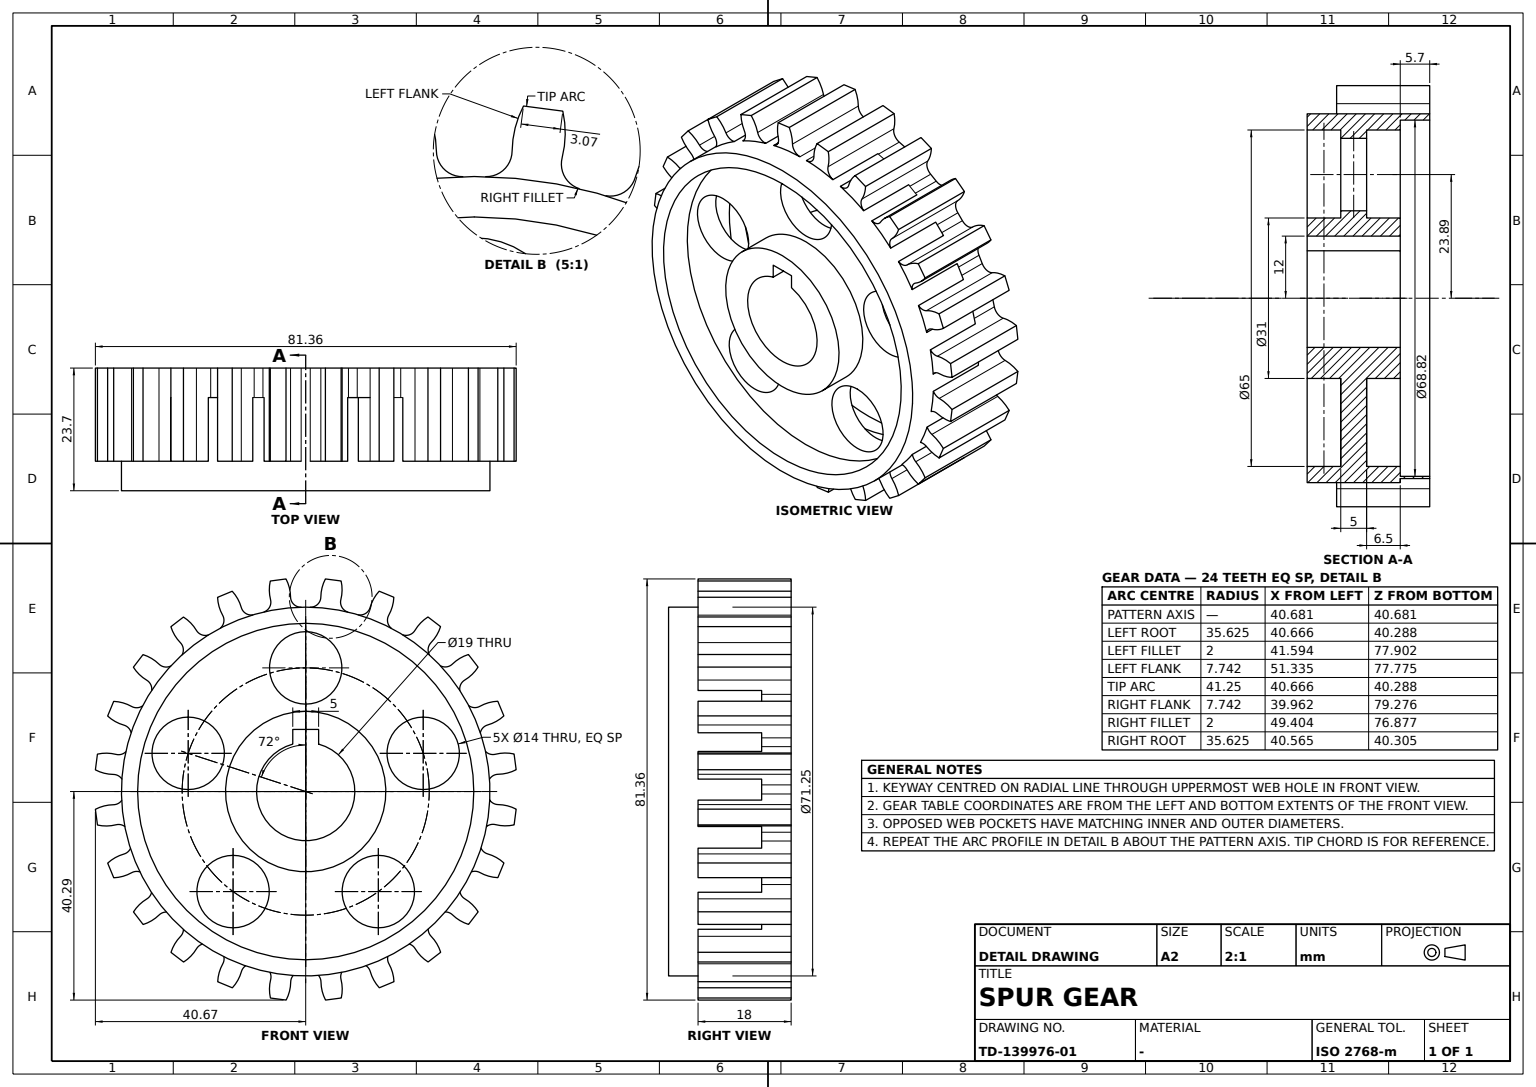
CATIA V5 part; units mm, degrees
sketch "Sketch1" plane through (0, 0, 0) normal (0, 1, 0) x (-1, 0, 0)
  point P0 (0, 9.5)
  line L0 (0, 9.5) -> (-5.7, 9.5)
  line L1 (-5.7, 9.5) -> (-5.7, 15.5)
  line L2 (-5.7, 15.5) -> (0.8, 15.5)
  line L3 (0.8, 15.5) -> (0.8, 32.5)
  line L4 (0.8, 32.5) -> (-5.7, 32.5)
  point P1 (-5.7, 32.5)
  line L5 (-5.7, 32.5) -> (-5.7, 35.625)
  line L6 (-5.7, 35.625) -> (12.3, 35.625)
  line L7 (12.3, 35.625) -> (12.3, 32.5)
  point P2 (12.3, 32.5)
  line L8 (12.3, 32.5) -> (5.8, 32.5)
  line L9 (5.8, 32.5) -> (5.8, 15.5)
  point P3 (5.8, 15.5)
  line L10 (5.8, 15.5) -> (12.3, 15.5)
  point P4 (12.3, 15.5)
  line L11 (12.3, 15.5) -> (12.3, 9.5)
  point P5 (12.3, 9.5)
  line L12 (12.3, 9.5) -> (0, 9.5)
  dimension "length L7" = 3.125
  dimension "length L11" = 6
  dimension "distance L1 y axis" = 5.7
  dimension "distance L3 L5" = 6.5
  dimension "distance L9 L3" = 5
  dimension "distance L5 L7" = 18
  dimension "distance L6 x axis" = 35.625
  dimension "distance L12 x axis" = 9.5
  constraint coincidence P0 y-axis
  constraint coincidence P1 L1
  constraint coincidence P2 L4
  constraint coincidence P3 L2
  constraint coincidence P4 L7
  constraint coincidence P5 L0
  constraint horizontal L0 x-axis
  constraint horizontal L2 x-axis
  constraint horizontal L4 x-axis
  constraint horizontal L6 x-axis
  constraint horizontal L8 x-axis
  constraint horizontal L10 x-axis
  constraint horizontal L12 x-axis
  constraint vertical L1 y-axis
  constraint vertical L3 y-axis
  constraint vertical L5 y-axis
  constraint vertical L7 y-axis
  constraint vertical L9 y-axis
  constraint vertical L11 y-axis
revolve "Shaft1" add sketch "Sketch1" angle 360 about axis through (0, 0, 0) along (-1, 0, 0)
sketch "Sketch2" plane through (0, 0, 0) normal (1, 0, 0) x (0, 1, 0)
  circle A0 centre (0, 23.89) radius 7
  point P0 (0, 23.89)
  circle A1 centre (-22.7207, 7.3824) radius 7
  circle A2 centre (-14.0422, -19.3274) radius 7
  circle A3 centre (14.0422, -19.3274) radius 7
  circle A4 centre (22.7207, 7.3824) radius 7
  circle A5 centre (0, 0) radius 9.5 construction
  arc A6 (2.5, 9.1652) -> (-2.5, 9.1652) centre (0, 0) ccw
  line L0 (-2.5, 12) -> (2.5, 12)
  line L1 (2.5, 12) -> (2.5, 9.1652)
  line L2 (-2.5, 9.1652) -> (-2.5, 12)
  point P1 (-2.5, 9.1652)
  dimension "radius A0" = 7
  dimension "distance P0 x axis" = 23.89
  dimension "distance L0 x axis" = 12
  dimension "length L0" = 5
  constraint coincidence P0 y-axis
  constraint coincidence P1 A5
  constraint horizontal L0 x-axis
  constraint vertical L1 y-axis
  constraint vertical L2 y-axis
  constraint symmetry L2 L1 y-axis
extrude "Pocket1" cut sketch "Sketch2" against normal through all and the other way up to next
sketch "Sketch3" plane through (0, 0, 0) normal (1, 0, 0) x (0, 1, 0)
  circle A0 centre (0, 0) radius 35.625 construction
  arc A1 (0.8787, 35.6142) -> (-0.8787, 35.6142) centre (0, 0) ccw
  circle A2 centre (0, 0) radius 34.411
  arc A3 (-2.9279, 37.5875) -> (-3.8084, 41.0738) centre (-10.669, 37.4868) ccw
  point P0 (-2.5164, 34.3189)
  point P1 (-6.4518, 33.8008)
  point P2 (-3.8084, 41.0738)
  point P3 (6.8509, 40.6771)
  point P4 (3.8084, 41.0738)
  arc A4 (3.8084, 41.0738) -> (6.8509, 40.6771) centre (0, 0) cw
  arc A5 (2.9279, 37.5875) -> (3.8084, 41.0738) centre (10.669, 37.4868) cw
  point P5 (-3.1914, 35.4818)
  point P6 (3.1914, 35.4818)
  arc A6 (-2.9279, 37.5875) -> (-0.8787, 35.6142) centre (-0.9281, 37.6136) ccw
  arc A7 (2.9279, 37.5875) -> (0.8787, 35.6142) centre (0.9281, 37.6136) cw
  point P7 (40.2989, -6.4434)
  point P8 (37.1569, -16.6368)
  point P9 (35.0987, -6.1007)
  point P10 (33.4468, -12.266)
  arc A8 (36.7035, -6.3916) -> (40.2989, -6.4434) centre (38.6097, 1.1119) ccw
  arc A9 (38.3275, -13.8006) -> (37.1569, -16.6368) centre (-0.3611, 0.5087) cw
  arc A10 (35.1879, -12.0478) -> (38.3275, -13.8006) centre (33.087, -19.4991) cw
  arc A11 (36.7035, -6.3916) -> (34.267, -7.8602) centre (36.211, -8.33) ccw
  arc A12 (35.1879, -12.0478) -> (33.8121, -9.5577) centre (35.7306, -10.1229) cw
  circle A13 centre (0, 0) radius 35.625 construction
  arc A14 (33.8121, -9.5577) -> (34.267, -7.8602) centre (-0.3611, 0.5087) ccw
  point P11 (-17.015, -36.7494)
  point P12 (-26.0479, -31.0762)
  point P13 (-14.9771, -32.3238)
  point P14 (-20.5047, -29.1324)
  arc A15 (-16.0344, -33.2899) -> (-17.015, -36.7494) centre (-9.28, -37.0732) ccw
  arc A16 (-23.6114, -32.941) -> (-26.0479, -31.0762) centre (0.2237, 0.7258) cw
  arc A17 (-21.1057, -30.362) -> (-23.6114, -32.941) centre (-27.7593, -26.4042) cw
  arc A18 (-16.0344, -33.2899) -> (-16.8224, -30.5563) centre (-17.7793, -32.3125) ccw
  arc A19 (-21.1057, -30.362) -> (-18.3444, -29.6776) centre (-19.3868, -31.3845) cw
  arc A20 (-18.3444, -29.6776) -> (-16.8224, -30.5563) centre (0.2237, 0.7258) ccw
  circle A21 centre (0, 0) radius 35.625 construction
  point P15 (-31.4544, 26.4554)
  point P16 (-23.6367, 33.7121)
  point P17 (-27.346, 22.8328)
  point P18 (-22.8328, 27.346)
  arc A22 (-28.3666, 24.6128) -> (-31.4544, 26.4554) centre (-33.7692, 19.0677) ccw
  arc A23 (-26.0686, 31.8412) -> (-23.6367, 33.7121) centre (0.2821, 0.1047) cw
  arc A24 (-24.226, 28.7535) -> (-26.0686, 31.8412) centre (-18.6809, 34.156) cw
  arc A25 (-28.3666, 24.6128) -> (-25.5223, 24.6664) centre (-26.971, 26.0453) ccw
  arc A26 (-24.226, 28.7535) -> (-24.2796, 25.9091) centre (-25.6585, 27.3578) cw
  arc A27 (-24.2796, 25.9091) -> (-25.5223, 24.6664) centre (0.2821, 0.1047) ccw
  circle A28 centre (0, 0) radius 35.625 construction
  point P19 (33.3339, 24.0442)
  point P20 (38.3199, 14.6146)
  point P21 (29.1324, 20.5047)
  point P22 (32.3238, 14.9771)
  arc A29 (30.7549, 21.5385) -> (33.3339, 24.0442) centre (26.7971, 28.1921) ccw
  arc A30 (37.1422, 17.4478) -> (38.3199, 14.6146) centre (-0.3329, 0.2091) cw
  arc A31 (33.6828, 16.4672) -> (37.1422, 17.4478) centre (37.4661, 9.7128) cw
  arc A32 (30.7549, 21.5385) -> (30.0705, 18.7772) centre (31.7773, 19.8196) ccw
  arc A33 (33.6828, 16.4672) -> (30.9492, 17.2552) centre (32.7054, 18.2121) cw
  arc A34 (30.9492, 17.2552) -> (30.0705, 18.7772) centre (-0.3329, 0.2091) ccw
  circle A35 centre (0, 0) radius 35.625 construction
  point P23 (14.2364, -37.9125)
  point P24 (3.8376, -40.2881)
  point P25 (12.266, -33.4468)
  point P26 (6.1007, -35.0987)
  arc A36 (12.4836, -34.7728) -> (14.2364, -37.9125) centre (19.9349, -32.672) ccw
  arc A37 (6.8791, -39.8838) -> (3.8376, -40.2881) centre (-0.0729, 0.7761) cw
  arc A38 (6.8273, -36.2884) -> (6.8791, -39.8838) centre (-0.6762, -38.1947) cw
  arc A39 (12.4836, -34.7728) -> (9.9935, -33.3971) centre (10.5586, -35.3156) ccw
  arc A40 (6.8273, -36.2884) -> (8.2959, -33.8519) centre (8.7657, -35.796) cw
  arc A41 (8.2959, -33.8519) -> (9.9935, -33.3971) centre (-0.0729, 0.7761) ccw
  circle A42 centre (0, 0) radius 35.625 construction
  point P27 (-40.6663, -3.4301)
  point P28 (-40.2696, 7.2291)
  point P29 (-35.4818, -3.1914)
  point P30 (-35.4818, 3.1914)
  arc A43 (-37.18, -2.5497) -> (-40.6663, -3.4301) centre (-37.0793, -10.2908) ccw
  arc A44 (-40.6663, 4.1866) -> (-40.2696, 7.2291) centre (0.4075, 0.3782) cw
  arc A45 (-37.18, 3.3061) -> (-40.6663, 4.1866) centre (-37.0793, 11.0473) cw
  arc A46 (-37.18, -2.5497) -> (-35.2067, -0.5005) centre (-37.2061, -0.5498) ccw
  arc A47 (-37.18, 3.3061) -> (-35.2067, 1.257) centre (-37.2061, 1.3063) cw
  arc A48 (-35.2067, 1.257) -> (-35.2067, -0.5005) centre (0.4075, 0.3782) ccw
  circle A49 centre (0, 0) radius 35.625 construction
  point P31 (6.8509, 40.6771)
  point P32 (17.0443, 37.5351)
  point P33 (6.1007, 35.0987)
  point P34 (12.266, 33.4468)
  arc A50 (6.7991, 37.0817) -> (6.8509, 40.6771) centre (-0.7044, 38.988) ccw
  arc A51 (14.2081, 38.7058) -> (17.0443, 37.5351) centre (-0.1012, 0.0172) cw
  arc A52 (12.4553, 35.5661) -> (14.2081, 38.7058) centre (19.9066, 33.4653) cw
  arc A53 (6.7991, 37.0817) -> (8.2676, 34.6452) centre (8.7375, 36.5893) ccw
  arc A54 (12.4553, 35.5661) -> (9.9652, 34.1904) centre (10.5304, 36.1089) cw
  arc A55 (9.9652, 34.1904) -> (8.2676, 34.6452) centre (-0.1012, 0.0172) ccw
  circle A56 centre (0, 0) radius 35.625 construction
  point P35 (37.1569, -16.6368)
  point P36 (31.4837, -25.6696)
  point P37 (32.3238, -14.9771)
  point P38 (29.1324, -20.5047)
  arc A57 (33.6974, -15.6562) -> (37.1569, -16.6368) centre (37.4807, -8.9018) ccw
  arc A58 (33.3485, -23.2331) -> (31.4837, -25.6696) centre (-0.3183, 0.602) cw
  arc A59 (30.7695, -20.7274) -> (33.3485, -23.2331) centre (26.8117, -27.3811) cw
  arc A60 (33.6974, -15.6562) -> (30.9638, -16.4441) centre (32.72, -17.4011) ccw
  arc A61 (30.7695, -20.7274) -> (30.0851, -17.9661) centre (31.792, -19.0085) cw
  arc A62 (30.0851, -17.9661) -> (30.9638, -16.4441) centre (-0.3183, 0.602) ccw
  circle A63 centre (0, 0) radius 35.625 construction
  point P39 (-26.0479, -31.0762)
  point P40 (-33.3046, -23.2584)
  point P41 (-22.8328, -27.346)
  point P42 (-27.346, -22.8328)
  arc A64 (-24.2053, -27.9884) -> (-26.0479, -31.0762) centre (-18.6602, -33.391) ccw
  arc A65 (-31.4338, -25.6903) -> (-33.3046, -23.2584) centre (0.3028, 0.6603) cw
  arc A66 (-28.346, -23.8477) -> (-31.4338, -25.6903) centre (-33.7485, -18.3027) cw
  arc A67 (-24.2053, -27.9884) -> (-24.2589, -25.1441) centre (-25.6378, -26.5927) ccw
  arc A68 (-28.346, -23.8477) -> (-25.5016, -23.9013) centre (-26.9503, -25.2802) cw
  arc A69 (-25.5016, -23.9013) -> (-24.2589, -25.1441) centre (0.3028, 0.6603) ccw
  circle A70 centre (0, 0) radius 35.625 construction
  point P43 (-23.6367, 33.7121)
  point P44 (-14.2071, 38.6982)
  point P45 (-20.5047, 29.1324)
  point P46 (-14.9771, 32.3238)
  arc A71 (-21.131, 31.1331) -> (-23.6367, 33.7121) centre (-27.7847, 27.1753) ccw
  arc A72 (-17.0404, 37.5205) -> (-14.2071, 38.6982) centre (0.1984, 0.0453) cw
  arc A73 (-16.0597, 34.061) -> (-17.0404, 37.5205) centre (-9.3053, 37.8443) cw
  arc A74 (-21.131, 31.1331) -> (-18.3697, 30.4487) centre (-19.4121, 32.1556) ccw
  arc A75 (-16.0597, 34.061) -> (-16.8477, 31.3275) centre (-17.8047, 33.0836) cw
  arc A76 (-16.8477, 31.3275) -> (-18.3697, 30.4487) centre (0.1984, 0.0453) ccw
  circle A77 centre (0, 0) radius 35.625 construction
  point P47 (38.3199, 14.6146)
  point P48 (40.6956, 4.2159)
  point P49 (33.4468, 12.266)
  point P50 (35.0987, 6.1007)
  arc A78 (35.1803, 12.8618) -> (38.3199, 14.6146) centre (33.0794, 20.3131) ccw
  arc A79 (40.2913, 7.2574) -> (40.6956, 4.2159) centre (-0.3686, 0.3053) cw
  arc A80 (36.6959, 7.2055) -> (40.2913, 7.2574) centre (38.6022, -0.2979) cw
  arc A81 (35.1803, 12.8618) -> (33.8046, 10.3717) centre (35.7231, 10.9369) ccw
  arc A82 (36.6959, 7.2055) -> (34.2594, 8.6741) centre (36.2035, 9.144) cw
  arc A83 (34.2594, 8.6741) -> (33.8046, 10.3717) centre (-0.3686, 0.3053) ccw
  circle A84 centre (0, 0) radius 35.625 construction
  point P51 (3.8376, -40.2881)
  point P52 (-6.8216, -39.8914)
  point P53 (3.1914, -35.4818)
  point P54 (-3.1914, -35.4818)
  arc A85 (2.9571, -36.8018) -> (3.8376, -40.2881) centre (10.6983, -36.701) ccw
  arc A86 (-3.7791, -40.2881) -> (-6.8216, -39.8914) centre (0.0292, 0.7857) cw
  arc A87 (-2.8987, -36.8018) -> (-3.7791, -40.2881) centre (-10.6398, -36.701) cw
  arc A88 (2.9571, -36.8018) -> (0.908, -34.8284) centre (0.9573, -36.8278) ccw
  arc A89 (-2.8987, -36.8018) -> (-0.8495, -34.8284) centre (-0.8988, -36.8278) cw
  arc A90 (-0.8495, -34.8284) -> (0.908, -34.8284) centre (0.0292, 0.7857) ccw
  circle A91 centre (0, 0) radius 35.625 construction
  point P55 (-40.2696, 7.2291)
  point P56 (-37.1276, 17.4225)
  point P57 (-35.0987, 6.1007)
  point P58 (-33.4468, 12.266)
  arc A92 (-36.6742, 7.1773) -> (-40.2696, 7.2291) centre (-38.5805, -0.3262) ccw
  arc A93 (-38.2983, 14.5864) -> (-37.1276, 17.4225) centre (0.3903, 0.2771) cw
  arc A94 (-35.1586, 12.8336) -> (-38.2983, 14.5864) centre (-33.0578, 20.2849) cw
  arc A95 (-36.6742, 7.1773) -> (-34.2378, 8.6459) centre (-36.1818, 9.1157) ccw
  arc A96 (-35.1586, 12.8336) -> (-33.7829, 10.3435) centre (-35.7014, 10.9086) cw
  arc A97 (-33.7829, 10.3435) -> (-34.2378, 8.6459) centre (0.3903, 0.2771) ccw
  circle A98 centre (0, 0) radius 35.625 construction
  point P59 (17.0443, 37.5351)
  point P60 (26.0771, 31.8619)
  point P61 (14.9771, 32.3238)
  point P62 (20.5047, 29.1324)
  arc A99 (16.0637, 34.0756) -> (17.0443, 37.5351) centre (9.3092, 37.859) ccw
  arc A100 (23.6406, 33.7267) -> (26.0771, 31.8619) centre (-0.1945, 0.0599) cw
  arc A101 (21.1349, 31.1477) -> (23.6406, 33.7267) centre (27.7886, 27.1899) cw
  arc A102 (16.0637, 34.0756) -> (16.8516, 31.3421) centre (17.8086, 33.0983) ccw
  arc A103 (21.1349, 31.1477) -> (18.3736, 30.4633) centre (19.416, 32.1702) cw
  arc A104 (18.3736, 30.4633) -> (16.8516, 31.3421) centre (-0.1945, 0.0599) ccw
  circle A105 centre (0, 0) radius 35.625 construction
  point P63 (31.4837, -25.6696)
  point P64 (23.6659, -32.9264)
  point P65 (27.346, -22.8328)
  point P66 (22.8328, -27.346)
  arc A106 (28.3959, -23.8271) -> (31.4837, -25.6696) centre (33.7985, -18.282) ccw
  arc A107 (26.0978, -31.0555) -> (23.6659, -32.9264) centre (-0.2528, 0.681) cw
  arc A108 (24.2552, -27.9677) -> (26.0978, -31.0555) centre (18.7102, -33.3703) cw
  arc A109 (28.3959, -23.8271) -> (25.5515, -23.8807) centre (27.0002, -25.2596) ccw
  arc A110 (24.2552, -27.9677) -> (24.3088, -25.1234) centre (25.6877, -26.572) cw
  arc A111 (24.3088, -25.1234) -> (25.5515, -23.8807) centre (-0.2528, 0.681) ccw
  circle A112 centre (0, 0) radius 35.625 construction
  point P67 (-33.3046, -23.2584)
  point P68 (-38.2907, -13.8289)
  point P69 (-29.1324, -20.5047)
  point P70 (-32.3238, -14.9771)
  arc A113 (-30.7256, -20.7528) -> (-33.3046, -23.2584) centre (-26.7678, -27.4064) ccw
  arc A114 (-37.113, -16.6621) -> (-38.2907, -13.8289) centre (0.3622, 0.5766) cw
  arc A115 (-33.6535, -15.6815) -> (-37.113, -16.6621) centre (-37.4369, -8.9271) cw
  arc A116 (-30.7256, -20.7528) -> (-30.0412, -17.9915) centre (-31.7481, -19.0339) ccw
  arc A117 (-33.6535, -15.6815) -> (-30.92, -16.4694) centre (-32.6762, -17.4264) cw
  arc A118 (-30.92, -16.4694) -> (-30.0412, -17.9915) centre (0.3622, 0.5766) ccw
  circle A119 centre (0, 0) radius 35.625 construction
  point P71 (-14.2071, 38.6982)
  point P72 (-3.8084, 41.0738)
  point P73 (-12.266, 33.4468)
  point P74 (-6.1007, 35.0987)
  arc A120 (-12.4543, 35.5586) -> (-14.2071, 38.6982) centre (-19.9056, 33.4577) ccw
  arc A121 (-6.8499, 40.6695) -> (-3.8084, 41.0738) centre (0.1022, 0.0096) cw
  arc A122 (-6.7981, 37.0742) -> (-6.8499, 40.6695) centre (0.7054, 38.9804) cw
  arc A123 (-12.4543, 35.5586) -> (-9.9642, 34.1828) centre (-10.5294, 36.1013) ccw
  arc A124 (-6.7981, 37.0742) -> (-8.2667, 34.6377) centre (-8.7365, 36.5817) cw
  arc A125 (-8.2667, 34.6377) -> (-9.9642, 34.1828) centre (0.1022, 0.0096) ccw
  circle A126 centre (0, 0) radius 35.625 construction
  point P75 (40.6956, 4.2159)
  point P76 (40.2989, -6.4434)
  point P77 (35.4818, 3.1914)
  point P78 (35.4818, -3.1914)
  arc A127 (37.2093, 3.3354) -> (40.6956, 4.2159) centre (37.1085, 11.0765) ccw
  arc A128 (40.6956, -3.4009) -> (40.2989, -6.4434) centre (-0.3782, 0.4075) cw
  arc A129 (37.2093, -2.5204) -> (40.6956, -3.4009) centre (37.1085, -10.2616) cw
  arc A130 (37.2093, 3.3354) -> (35.2359, 1.2862) centre (37.2353, 1.3356) ccw
  arc A131 (37.2093, -2.5204) -> (35.2359, -0.4712) centre (37.2353, -0.5206) cw
  arc A132 (35.2359, -0.4712) -> (35.2359, 1.2862) centre (-0.3782, 0.4075) ccw
  circle A133 centre (0, 0) radius 35.625 construction
  point P79 (-6.8216, -39.8914)
  point P80 (-17.015, -36.7494)
  point P81 (-6.1007, -35.0987)
  point P82 (-12.266, -33.4468)
  arc A134 (-6.7698, -36.296) -> (-6.8216, -39.8914) centre (0.7336, -38.2022) ccw
  arc A135 (-14.1789, -37.92) -> (-17.015, -36.7494) centre (0.1304, 0.7686) cw
  arc A136 (-12.4261, -34.7804) -> (-14.1789, -37.92) centre (-19.8774, -32.6795) cw
  arc A137 (-6.7698, -36.296) -> (-8.2384, -33.8595) centre (-8.7082, -35.8035) ccw
  arc A138 (-12.4261, -34.7804) -> (-9.936, -33.4046) centre (-10.5011, -35.3231) cw
  arc A139 (-9.936, -33.4046) -> (-8.2384, -33.8595) centre (0.1304, 0.7686) ccw
  circle A140 centre (0, 0) radius 35.625 construction
  point P83 (-37.1276, 17.4225)
  point P84 (-31.4544, 26.4554)
  point P85 (-32.3238, 14.9771)
  point P86 (-29.1324, 20.5047)
  arc A141 (-33.6682, 16.4419) -> (-37.1276, 17.4225) centre (-37.4515, 9.6875) ccw
  arc A142 (-33.3192, 24.0188) -> (-31.4544, 26.4554) centre (0.3475, 0.1838) cw
  arc A143 (-30.7403, 21.5132) -> (-33.3192, 24.0188) centre (-26.7824, 28.1668) cw
  arc A144 (-33.6682, 16.4419) -> (-30.9346, 17.2298) centre (-32.6908, 18.1868) ccw
  arc A145 (-30.7403, 21.5132) -> (-30.0559, 18.7519) centre (-31.7627, 19.7943) cw
  arc A146 (-30.0559, 18.7519) -> (-30.9346, 17.2298) centre (0.3475, 0.1838) ccw
  circle A147 centre (0, 0) radius 35.625 construction
  point P87 (26.0771, 31.8619)
  point P88 (33.3339, 24.0442)
  point P89 (22.8328, 27.346)
  point P90 (27.346, 22.8328)
  arc A148 (24.2345, 28.7741) -> (26.0771, 31.8619) centre (18.6895, 34.1767) ccw
  arc A149 (31.463, 26.476) -> (33.3339, 24.0442) centre (-0.2735, 0.1254) cw
  arc A150 (28.3752, 24.6335) -> (31.463, 26.476) centre (33.7778, 19.0884) cw
  arc A151 (24.2345, 28.7741) -> (24.2881, 25.9298) centre (25.667, 27.3784) ccw
  arc A152 (28.3752, 24.6335) -> (25.5309, 24.6871) centre (26.9795, 26.066) cw
  arc A153 (25.5309, 24.6871) -> (24.2881, 25.9298) centre (-0.2735, 0.1254) ccw
  circle A154 centre (0, 0) radius 35.625 construction
  point P91 (23.6659, -32.9264)
  point P92 (14.2364, -37.9125)
  point P93 (20.5047, -29.1324)
  point P94 (14.9771, -32.3238)
  arc A155 (21.1602, -30.3474) -> (23.6659, -32.9264) centre (27.8139, -26.3896) ccw
  arc A156 (17.0696, -36.7348) -> (14.2364, -37.9125) centre (-0.1691, 0.7404) cw
  arc A157 (16.089, -33.2753) -> (17.0696, -36.7348) centre (9.3346, -37.0586) cw
  arc A158 (21.1602, -30.3474) -> (18.3989, -29.663) centre (19.4414, -31.3699) ccw
  arc A159 (16.089, -33.2753) -> (16.8769, -30.5417) centre (17.8339, -32.2979) cw
  arc A160 (16.8769, -30.5417) -> (18.3989, -29.663) centre (-0.1691, 0.7404) ccw
  circle A161 centre (0, 0) radius 35.625 construction
  point P95 (-38.2907, -13.8289)
  point P96 (-40.6663, -3.4301)
  point P97 (-33.4468, -12.266)
  point P98 (-35.0987, -6.1007)
  arc A162 (-35.1511, -12.0761) -> (-38.2907, -13.8289) centre (-33.0502, -19.5274) ccw
  arc A163 (-40.2621, -6.4716) -> (-40.6663, -3.4301) centre (0.3979, 0.4804) cw
  arc A164 (-36.6667, -6.4198) -> (-40.2621, -6.4716) centre (-38.5729, 1.0836) cw
  arc A165 (-35.1511, -12.0761) -> (-33.7753, -9.586) centre (-35.6938, -10.1511) ccw
  arc A166 (-36.6667, -6.4198) -> (-34.2302, -7.8884) centre (-36.1742, -8.3582) cw
  arc A167 (-34.2302, -7.8884) -> (-33.7753, -9.586) centre (0.3979, 0.4804) ccw
  circle A168 centre (0, 0) radius 35.625 construction
  dimension "radius A2" = 34.411
  dimension "radius A6" = 2
  dimension "radius A7" = 2
  constraint coincidence A2 P0
  constraint coincidence A2 P1
  constraint coincidence A0 P5
  constraint coincidence A0 P6
  constraint coincidence A3 P5
  constraint coincidence A5 P6
  constraint coincidence P2 P72
  constraint coincidence P3 P31
  constraint coincidence P32 A99
  constraint coincidence P32 P59
  constraint coincidence P60 P87
  constraint coincidence P88 P19
  constraint coincidence P20 P47
  constraint coincidence P48 P75
  constraint coincidence P76 P7
  constraint coincidence P8 P35
  constraint coincidence P36 P63
  constraint coincidence P64 P91
  constraint coincidence P92 P23
  constraint coincidence P51 P24
  constraint coincidence P52 P79
  constraint coincidence P11 P80
  constraint coincidence P39 P12
  constraint coincidence P40 P67
  constraint coincidence P95 P68
  constraint coincidence P27 P96
  constraint coincidence P55 P28
  constraint coincidence P83 P56
  constraint coincidence P84 P15
  constraint coincidence P16 P43
  constraint coincidence P44 P71
  constraint symmetry P2 P4 y-axis
  constraint symmetry A3 A5 y-axis
  constraint tangency A6 A3
  constraint tangency A6 A0
  constraint tangency A7 A5
  constraint tangency A7 A0
extrude "Pad1" add sketch "Sketch3" against normal blind 18
sketch "Sketch4" plane through (0, 0, 0) normal (0, 0, 1) x (1, 0, 0)
